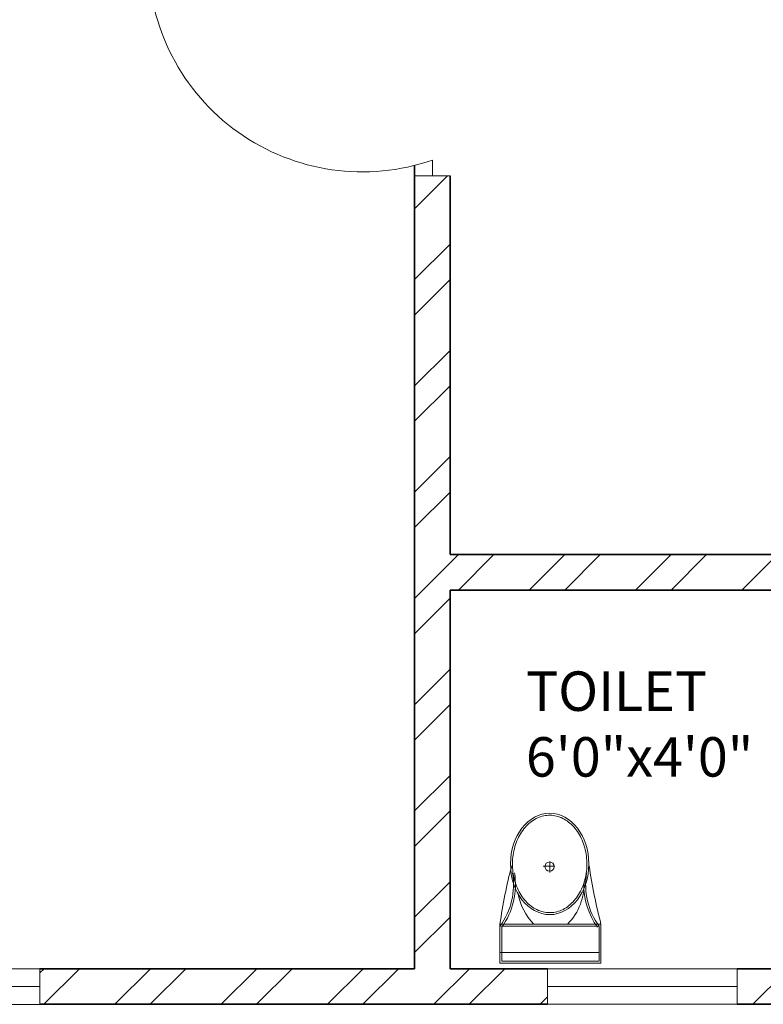
# Model space of a CAD drawing. Units: inches. Extents: x 1885 to 2748, y 783 to 2421.
# Tile 42 of 117: x 2098 to 2192, y 1558 to 1683. Entities that reach past the tile are written whole.
import ezdxf

# ---------------------------------------------------------------- set-up
doc = ezdxf.new("R2010")
doc.units = ezdxf.units.IN
for name, color, linetype, lineweight in [('A-AREA-IDEN', 7, 'Continuous', 18), ('A-DOOR', 31, 'Continuous', 18), ('A-FLOR-FIXT', 8, 'Continuous', 18), ('A-GLAZ', 181, 'Continuous', 18), ('A-WALL', 7, 'Continuous', 35)]:
    doc.layers.add(name, color=color, linetype=linetype, lineweight=lineweight)
doc.layers.add('A-WALL-PATT', color=85, linetype='Continuous', lineweight=13, true_color=0x58ba48)
doc.styles.get("Standard").update_dxf_attribs({"font": 'arial.ttf'})

# ---------------------------------------------------------------- blocks, each defined once
blk = doc.blocks.new('A$C31115884')
for p, q in [((257.5, 466.4), (257.5, 523.2)), ((283.1, 497.7), (223.4, 497.7)), ((0, 200), (0, 0)), ((520, 200), (0, 200)), ((10, 190), (10, 10)), ((510, 190), (10, 190)), ((510, 10), (510, 190)), ((520, 0), (520, 200)), ((510, 54.5), (0, 54.5)), ((10, 10), (510, 10)), ((0, 0), (520, 0))]:
    blk.add_line(p, q)
blk.add_circle((255.6, 496.4), 23.6)
for centre, radius, start, end in [((2777.7, -204.6), 2807, 165.4549, 171.7133), ((-294.5, 403.3), 364.7, 324.2091, 9.3499), ((-294.5, 403.3), 374.7, 324.2091, 9.3499), ((805.8, 403.3), 364.7, 170.6501, 215.7909), ((3237, 905), 2807, 188.2867, 194.5451), ((139.5, 406.2), 293.5, 315.8436, 2.6563), ((805.8, 403.3), 374.7, 179.2036, 215.7909), ((383.6, 406.2), 293.5, 190.2774, 224.1564)]:
    blk.add_arc(centre, radius, start, end)
blk.add_ellipse((256.2, 509.9), major_axis=(0, -260.7), ratio=0.772727)
blk.add_open_spline([(256.2, 259.2), (263.1, 259.2), (270, 259.7), (287.8, 262.3), (298.7, 265.1), (319.9, 273.1), (330.2, 278.4), (350.1, 291.1), (359.7, 298.7), (377.7, 315.9), (386.2, 325.5), (401.7, 346.6), (408.8, 358.1), (421.3, 382.5), (426.8, 395.5), (435.9, 422.4), (439.5, 436.4), (444.8, 465.1), (446.5, 479.7), (447.9, 509.2), (447.6, 524), (445, 553.3), (442.7, 567.8), (436.3, 596), (432.1, 609.7), (421.9, 636), (416, 648.6), (402.5, 672.1), (395, 683), (378.6, 703), (369.8, 712.1), (351.1, 728), (341.3, 734.8), (320.9, 746.2), (310.4, 750.7), (288.9, 757.3), (278, 759.4), (256, 761), (245, 760.6), (223.1, 757.2), (212.3, 754.3), (191.1, 746.1), (180.8, 740.7), (160.9, 727.8), (151.4, 720.1), (133.5, 702.7), (125.1, 693), (109.6, 671.7), (102.6, 660.2), (90.2, 635.7), (84.9, 622.7), (76, 595.6), (72.4, 581.6), (67.2, 552.9), (65.6, 538.2), (64.4, 508.8), (64.8, 494), (67.5, 464.7), (69.9, 450.2), (76.6, 422), (80.8, 408.3), (91.1, 382.2), (97.2, 369.7), (110.8, 346.3), (118.4, 335.4), (134.8, 315.6), (143.7, 306.7), (162.4, 290.9), (172.3, 284.2), (192.8, 273), (203.3, 268.6), (224.8, 262.2), (235.8, 260.2), (249.9, 259.3), (253, 259.2), (256.2, 259.2)], degree=3, knots=[0, 0, 0, 0, 0.110105, 0.110105, 0.285049, 0.285049, 0.459994, 0.459994, 0.634938, 0.634938, 0.809882, 0.809882, 0.984827, 0.984827, 1.159771, 1.159771, 1.334715, 1.334715, 1.50966, 1.50966, 1.684604, 1.684604, 1.859549, 1.859549, 2.034493, 2.034493, 2.209437, 2.209437, 2.384382, 2.384382, 2.559326, 2.559326, 2.73427, 2.73427, 2.909215, 2.909215, 3.084159, 3.084159, 3.259103, 3.259103, 3.434048, 3.434048, 3.608992, 3.608992, 3.783936, 3.783936, 3.958881, 3.958881, 4.133825, 4.133825, 4.30877, 4.30877, 4.483714, 4.483714, 4.658658, 4.658658, 4.833603, 4.833603, 5.008547, 5.008547, 5.183491, 5.183491, 5.358436, 5.358436, 5.53338, 5.53338, 5.708324, 5.708324, 5.883269, 5.883269, 6.058213, 6.058213, 6.233158, 6.233158, 6.283185, 6.283185, 6.283185, 6.283185])
blk = doc.blocks.new('WIN-60')
for p, q in [((0, 60), (4.5, 60)), ((0, 60), (0, 0)), ((4.5, 60), (2.25, 60)), ((2.25, 60), (2.25, 0)), ((4.5, 0), (4.5, 60)), ((2.25, 0), (0, 0)), ((0, 0), (4.5, 0))]:
    blk.add_line(p, q)
blk = doc.blocks.new('WIN-24')
for p, q in [((0, 4.5), (0, 0)), ((0, 4.5), (24, 4.5)), ((24, 2.25), (24, 4.5)), ((24, 4.5), (24, 0)), ((0, 0), (0, 2.25)), ((0, 2.25), (24, 2.25)), ((24, 0), (0, 0))]:
    blk.add_line(p, q)

msp = doc.modelspace()

# ---------------------------------------------------------------- hatches: boundary and pattern name
at = {"layer": 'A-WALL-PATT'}
h = msp.add_hatch(dxfattribs=at)
h.set_pattern_fill('ANSI32', color=256)
h.paths.add_polyline_path([(2007.77, 2318.01), (1980.77, 2318.01), (1980.77, 2281.22), (1985.27, 2281.22), (1985.27, 2313.51), (2007.77, 2313.51), (2007.77, 2315.76)])
h.paths.add_polyline_path([(2094.32, 2318.01), (2067.77, 2318.01), (2067.77, 2313.51), (2094.32, 2313.51), (2094.32, 2315.76)])
h.paths.add_polyline_path([(2131.37, 2315.76), (2131.37, 2318.01), (2131.19, 2318.01), (2112.61, 2318.01), (2112.61, 2313.51), (2117.27, 2313.51), (2117.27, 2255.2), (2121.77, 2255.2), (2121.77, 2313.51), (2131.37, 2313.51)])
h.paths.add_polyline_path([(2190.51, 2318.01), (2155.37, 2318.01), (2155.37, 2313.51), (2169.77, 2313.51), (2169.77, 2229.51), (2121.77, 2229.51), (2121.77, 2233.45), (2119.52, 2233.45), (2117.27, 2233.45), (2117.27, 2201.1), (2121.77, 2201.1), (2121.77, 2225.01), (2169.77, 2225.01), (2169.77, 2165.01), (2306.27, 2165.01), (2306.27, 2066.01), (2310.77, 2066.01), (2344.27, 2066.01), (2486.27, 2066.01), (2486.27, 1886.01), (2483.02, 1886.01), (2483.02, 1881.51), (2486.27, 1881.51), (2486.27, 1880.68), (2490.77, 1880.68), (2490.77, 2070.51), (2344.27, 2070.51), (2310.77, 2070.51), (2310.77, 2165.01), (2310.77, 2173.64), (2308.52, 2173.64), (2306.27, 2173.64), (2306.27, 2169.51), (2174.27, 2169.51), (2174.27, 2313.51), (2190.51, 2313.51), (2190.51, 2315.76)])
h.paths.add_polyline_path([(1985.27, 2221.22), (1980.77, 2221.22), (1980.77, 2165.01), (1992.77, 2165.01), (1992.77, 2141.93), (1997.27, 2141.93), (1997.27, 2165.01), (2117.27, 2165.01), (2117.27, 2163.13), (2121.77, 2163.13), (2121.77, 2172.73), (2119.52, 2172.73), (2117.27, 2172.73), (2117.27, 2169.51), (1985.27, 2169.51)])
h.paths.add_polyline_path([(1997.27, 2105.93), (1992.77, 2105.93), (1992.77, 2070.51), (2016.77, 2070.51), (2016.77, 2059.12), (2019.02, 2059.12), (2021.27, 2059.12), (2021.27, 2070.51), (2117.27, 2070.51), (2117.27, 2022.51), (2114.42, 2022.51), (2114.42, 2018.01), (2123.63, 2018.01), (2123.63, 2020.26), (2123.63, 2022.51), (2121.77, 2022.51), (2121.77, 2142.59), (2119.52, 2142.59), (2117.27, 2142.59), (2117.27, 2075.01), (1997.27, 2075.01)])
h.paths.add_polyline_path([(2092.03, 2020.26), (2092.03, 2022.51), (2021.27, 2022.51), (2021.27, 2035.12), (2016.77, 2035.12), (2016.77, 2018.01), (2016.77, 1978.78), (2021.27, 1978.78), (2021.27, 2018.01), (2092.03, 2018.01)])
h.paths.add_polyline_path([(2260.94, 2022.51), (2153.1, 2022.51), (2153.1, 2020.26), (2153.1, 2018.01), (2155.27, 2018.01), (2155.27, 1886.01), (2107.63, 1886.01), (2107.63, 1881.51), (2182.91, 1881.51), (2182.91, 1883.76), (2182.91, 1886.01), (2159.77, 1886.01), (2159.77, 2018.01), (2260.94, 2018.01), (2260.94, 2020.26)])
h.paths.add_polyline_path([(2047.63, 1883.76), (2047.63, 1886.01), (2021.27, 1886.01), (2021.27, 1918.78), (2019.02, 1918.78), (2016.77, 1918.78), (2016.77, 1881.51), (2047.63, 1881.51)])
h.paths.add_polyline_path([(2306.36, 1883.76), (2306.36, 1886.01), (2296.27, 1886.01), (2296.27, 1982.01), (2316.54, 1982.01), (2316.54, 1984.26), (2316.54, 1986.51), (2296.27, 1986.51), (2296.27, 2022.51), (2289.28, 2022.51), (2289.28, 2018.01), (2291.77, 2018.01), (2291.77, 1886.01), (2242.91, 1886.01), (2242.91, 1881.51), (2306.36, 1881.51)], flags=17)
h.paths.add_polyline_path([(1985.27, 1843.01), (2021.6, 1843.01), (2021.53, 1845.44), (2021.48, 1847.51), (1980.77, 1847.51), (1980.77, 1809.45), (1985.27, 1809.45)])
h.paths.add_polyline_path([(2131.48, 1845.26), (2131.48, 1847.51), (2081.53, 1847.51), (2081.53, 1843.01), (2117.27, 1843.01), (2117.27, 1784.15), (2119.52, 1784.15), (2121.77, 1784.15), (2121.77, 1843.01), (2131.48, 1843.01)])
h.paths.add_polyline_path([(2203.89, 1847.51), (2155.48, 1847.51), (2155.48, 1843.01), (2169.77, 1843.01), (2169.77, 1759.01), (2121.77, 1759.01), (2121.77, 1761.46), (2117.27, 1761.46), (2117.27, 1730.43), (2121.77, 1730.43), (2121.77, 1754.51), (2177.42, 1754.51), (2177.42, 1756.76), (2177.42, 1759.01), (2174.27, 1759.01), (2174.27, 1843.01), (2203.89, 1843.01)])
h.paths.add_polyline_path([(2335.55, 1845.26), (2335.55, 1847.51), (2239.89, 1847.51), (2239.89, 1843.01), (2306.27, 1843.01), (2306.27, 1759.01), (2199.49, 1759.01), (2199.49, 1754.51), (2310.77, 1754.51), (2310.77, 1843.01), (2335.55, 1843.01)])
h.paths.add_polyline_path([(2348.77, 2022.51), (2344.27, 2022.51), (2344.27, 1986.51), (2341.68, 1986.51), (2341.68, 1982.01), (2344.27, 1982.01), (2344.27, 1886.01), (2330.36, 1886.01), (2330.36, 1881.51), (2361.63, 1881.51), (2361.63, 1883.76), (2361.63, 1886.01), (2348.77, 1886.01)], flags=17)
h.paths.add_polyline_path([(2283.25, 2315.76), (2283.25, 2318.01), (2238.51, 2318.01), (2238.51, 2313.51), (2283.25, 2313.51)], flags=17)
h.paths.add_polyline_path([(2363.27, 2348.01), (2388.68, 2348.01), (2388.68, 2350.26), (2388.68, 2352.51), (2358.77, 2352.51), (2358.77, 2348.01), (2358.77, 2318.01), (2344.48, 2318.01), (2344.48, 2313.51), (2358.77, 2313.51), (2358.77, 2229.51), (2310.77, 2229.51), (2310.77, 2231.95), (2306.27, 2231.95), (2306.27, 2205.61), (2310.77, 2205.61), (2310.77, 2225.01), (2358.77, 2225.01), (2358.77, 2211.51), (2452.33, 2211.51), (2452.33, 2213.76), (2452.33, 2216.01), (2363.27, 2216.01), (2363.27, 2318.01)])
h.paths.add_polyline_path([(2310.77, 2313.51), (2320.48, 2313.51), (2320.48, 2315.76), (2320.48, 2318.01), (2302.73, 2318.01), (2302.73, 2313.51), (2306.27, 2313.51), (2306.27, 2251.08), (2310.77, 2251.08)], flags=17)
h.paths.add_polyline_path([(2490.77, 2352.51), (2486.27, 2352.51), (2448.68, 2352.51), (2448.68, 2348.01), (2486.27, 2348.01), (2486.27, 2318.01), (2486.27, 2216.01), (2481.78, 2216.01), (2481.78, 2211.51), (2486.27, 2211.51), (2486.27, 2165.01), (2493.29, 2165.01), (2493.29, 2167.26), (2493.29, 2169.51), (2490.77, 2169.51), (2490.77, 2313.51), (2494.43, 2313.51), (2494.43, 2318.01), (2490.77, 2318.01)])
h.paths.add_polyline_path([(2534.65, 2318.01), (2515.69, 2318.01), (2515.69, 2313.51), (2534.65, 2313.51), (2534.65, 2315.76)])
h.paths.add_polyline_path([(2618.27, 2318.01), (2594.65, 2318.01), (2594.65, 2313.51), (2613.77, 2313.51), (2613.77, 2281.71), (2618.27, 2281.71)])
h.paths.add_polyline_path([(2618.27, 2221.71), (2613.77, 2221.71), (2613.77, 2169.51), (2554.02, 2169.51), (2554.02, 2165.01), (2613.77, 2165.01), (2613.77, 2152.88), (2618.27, 2152.88)])
h.paths.add_polyline_path([(2618.27, 2128.88), (2616.02, 2128.88), (2613.77, 2128.88), (2613.77, 2117.01), (2529.77, 2117.01), (2529.77, 2165.01), (2532.85, 2165.01), (2532.85, 2169.51), (2522.87, 2169.51), (2522.87, 2165.01), (2525.27, 2165.01), (2525.27, 2117.01), (2525.27, 2112.51), (2525.27, 2108.58), (2529.77, 2108.58), (2529.77, 2112.51), (2613.77, 2112.51), (2613.77, 2080.19), (2618.27, 2080.19)])
h.paths.add_polyline_path([(2618.27, 2044.19), (2616.02, 2044.19), (2613.77, 2044.19), (2613.77, 2015.51), (2529.77, 2015.51), (2529.77, 2088.58), (2527.52, 2088.58), (2525.27, 2088.58), (2525.27, 2011.01), (2613.77, 2011.01), (2613.77, 1956.75), (2618.27, 1956.75)])
h.paths.add_polyline_path([(2618.27, 1881.51), (2618.27, 1896.75), (2613.77, 1896.75), (2613.77, 1881.51), (2613.77, 1847.51), (2592.71, 1847.51), (2592.71, 1843.01), (2613.77, 1843.01), (2613.77, 1765.01), (2613.77, 1760.51), (2609.62, 1760.51), (2609.62, 1756.01), (2613.77, 1756.01), (2613.77, 1660.01), (2608.54, 1660.01), (2608.54, 1655.51), (2613.77, 1655.51), (2613.77, 1508.16), (2618.27, 1508.16)])
h.paths.add_polyline_path([(2565.77, 1843.01), (2569, 1843.01), (2569, 1847.51), (2490.77, 1847.51), (2490.77, 1849.7), (2488.52, 1849.7), (2486.27, 1849.7), (2486.27, 1847.51), (2477.27, 1847.51), (2477.27, 1838.51), (2477.27, 1821.49), (2486.27, 1821.49), (2486.27, 1838.51), (2561.27, 1838.51), (2561.27, 1765.01), (2486.27, 1765.01), (2486.27, 1786.16), (2477.27, 1786.16), (2477.27, 1765.01), (2477.27, 1756.01), (2486.27, 1756.01), (2565.77, 1756.01), (2585.62, 1756.01), (2585.62, 1758.26), (2585.62, 1760.51), (2565.77, 1760.51), (2565.77, 1765.01)])
h.paths.add_polyline_path([(2486.27, 1651.01), (2561.27, 1651.01), (2561.27, 1567.01), (2486.27, 1567.01), (2486.27, 1591.32), (2477.27, 1591.32), (2477.27, 1567.01), (2477.27, 1558.01), (2477.27, 1555.44), (2481.77, 1555.44), (2481.77, 1558.01), (2568.65, 1558.01), (2568.65, 1560.26), (2568.65, 1562.51), (2565.77, 1562.51), (2565.77, 1655.51), (2584.54, 1655.51), (2584.54, 1657.76), (2584.54, 1660.01), (2565.77, 1660.01), (2486.27, 1660.01), (2477.27, 1660.01), (2477.27, 1651.01), (2477.27, 1632.99), (2486.27, 1632.99)])
h.paths.add_polyline_path([(2449.97, 1883.76), (2449.97, 1886.01), (2421.63, 1886.01), (2421.63, 1881.51), (2449.97, 1881.51)], flags=17)
h.paths.add_polyline_path([(2447.27, 1847.51), (2395.55, 1847.51), (2395.55, 1843.01), (2442.77, 1843.01), (2442.77, 1809.27), (2447.27, 1809.27)])
h.paths.add_polyline_path([(1985.27, 1749.45), (1980.77, 1749.45), (1980.77, 1694.5), (1985.27, 1694.5), (1985.27, 1694.51), (1986.9, 1694.51), (1986.9, 1697.78), (1986.9, 1699.01), (1985.27, 1699.01)])
h.paths.add_polyline_path([(2152.77, 1699.01), (2121.77, 1699.01), (2121.77, 1703.67), (2119.52, 1703.67), (2117.27, 1703.67), (2117.27, 1699.01), (2009.22, 1699.01), (2009.22, 1694.51), (2148.27, 1694.51), (2148.27, 1692.63), (2152.77, 1692.63)])
h.paths.add_polyline_path([(2016.27, 1694.51), (2011.77, 1694.51), (2011.77, 1558.01), (2040.81, 1558.01), (2040.81, 1560.26), (2040.81, 1562.51), (2016.27, 1562.51)])
h.paths.add_polyline_path([(2152.77, 1663.02), (2150.52, 1663.02), (2148.27, 1663.02), (2148.27, 1562.51), (2100.81, 1562.51), (2100.81, 1558.01), (2165.12, 1558.01), (2165.12, 1560.26), (2165.12, 1562.51), (2152.77, 1562.51), (2152.77, 1610.51), (2224.77, 1610.51), (2224.77, 1607.99), (2229.27, 1607.99), (2229.27, 1615.01), (2152.77, 1615.01)])
h.paths.add_polyline_path([(2238.61, 1560.26), (2238.61, 1562.51), (2229.27, 1562.51), (2229.27, 1588.76), (2227.02, 1588.76), (2224.77, 1588.77), (2224.77, 1562.51), (2189.12, 1562.51), (2189.12, 1558.01), (2238.61, 1558.01)])
h.paths.add_polyline_path([(2336.02, 1560.26), (2336.02, 1562.51), (2310.77, 1562.51), (2310.77, 1656.35), (2308.52, 1656.35), (2306.27, 1656.35), (2306.27, 1562.51), (2286.61, 1562.51), (2286.61, 1558.01), (2336.02, 1558.01)])
h.paths.add_polyline_path([(2447.27, 1690.97), (2445.02, 1690.97), (2442.77, 1690.97), (2442.77, 1687.01), (2306.27, 1687.01), (2306.27, 1680.75), (2310.77, 1680.75), (2310.77, 1682.51), (2442.77, 1682.51), (2442.77, 1562.51), (2396.02, 1562.51), (2396.02, 1558.01), (2447.27, 1558.01)])
h.paths.add_polyline_path([(2447.27, 1749.27), (2445.02, 1749.27), (2442.77, 1749.27), (2442.77, 1717.23), (2447.27, 1717.23)])
h.paths.add_polyline_path([(2044.67, 1521.76), (2044.67, 1524.01), (2007.27, 1524.01), (2007.27, 1503.49), (2009.52, 1503.49), (2011.77, 1503.49), (2011.77, 1519.51), (2044.67, 1519.51)])
h.paths.add_polyline_path([(2177.97, 1521.76), (2177.97, 1524.01), (2104.67, 1524.01), (2104.67, 1519.51), (2145.77, 1519.51), (2145.77, 1387.51), (2143.37, 1387.51), (2143.37, 1383.01), (2251.59, 1383.01), (2251.59, 1385.26), (2251.59, 1387.51), (2150.27, 1387.51), (2150.27, 1519.51), (2177.97, 1519.51)])
h.paths.add_polyline_path([(2298.7, 1524.01), (2237.97, 1524.01), (2237.97, 1519.51), (2282.27, 1519.51), (2282.27, 1387.51), (2279.68, 1387.51), (2279.68, 1383.01), (2286.77, 1383.01), (2286.77, 1419.01), (2312.45, 1419.01), (2312.45, 1421.26), (2312.45, 1423.51), (2286.77, 1423.51), (2286.77, 1519.51), (2298.7, 1519.51), (2298.7, 1521.72)], flags=17)
h.paths.add_polyline_path([(2361.9, 1521.76), (2361.9, 1524.01), (2322.7, 1524.01), (2322.7, 1519.51), (2334.77, 1519.51), (2334.77, 1423.51), (2331.93, 1423.51), (2331.93, 1419.01), (2334.77, 1419.01), (2334.77, 1387.51), (2334.77, 1383.23), (2339.27, 1383.23), (2339.27, 1387.51), (2339.27, 1519.51), (2361.9, 1519.51)], flags=17)
h.paths.add_polyline_path([(2447.27, 1521.76), (2447.27, 1524.01), (2421.9, 1524.01), (2421.9, 1519.51), (2447.27, 1519.51)], flags=17)
h.paths.add_polyline_path([(2481.77, 1529.6), (2479.52, 1529.6), (2477.27, 1529.6), (2477.27, 1524.01), (2474.49, 1524.01), (2474.49, 1519.51), (2477.27, 1519.51), (2477.27, 1334.51), (2296.77, 1334.51), (2296.77, 1240.51), (2160.27, 1240.51), (2160.27, 1180.51), (2112.27, 1180.51), (2112.27, 1207.69), (2110.02, 1207.69), (2107.77, 1207.69), (2107.77, 1171.61), (2112.27, 1171.61), (2112.27, 1176.01), (2160.27, 1176.01), (2160.27, 1092.01), (2144.22, 1092.01), (2144.22, 1087.51), (2189.5, 1087.51), (2189.5, 1089.76), (2189.5, 1092.01), (2164.77, 1092.01), (2164.77, 1236.01), (2296.77, 1236.01), (2296.77, 1231.91), (2301.27, 1231.91), (2301.27, 1330.01), (2481.77, 1330.01), (2481.77, 1387.51)])
h.paths.add_polyline_path([(2618.27, 1448.16), (2613.77, 1448.16), (2613.77, 1382.51), (2529.77, 1382.51), (2525.27, 1382.51), (2525.27, 1307.06), (2529.77, 1307.06), (2529.77, 1378.01), (2613.77, 1378.01), (2613.77, 1354.99), (2618.27, 1354.99)])
h.paths.add_polyline_path([(2618.27, 1318.99), (2613.77, 1318.99), (2613.77, 1281.01), (2529.77, 1281.01), (2529.77, 1283.79), (2527.52, 1283.79), (2525.27, 1283.79), (2525.27, 1228.51), (2516.79, 1228.51), (2516.79, 1224.01), (2533.48, 1224.01), (2533.48, 1226.26), (2533.48, 1228.51), (2529.77, 1228.51), (2529.77, 1276.51), (2613.77, 1276.51), (2613.77, 1266.02), (2618.27, 1266.02)])
h.paths.add_polyline_path([(2618.27, 1134.96), (2613.77, 1134.96), (2613.77, 1092.01), (2594.54, 1092.01), (2594.54, 1087.51), (2618.27, 1087.51)])
h.paths.add_polyline_path([(2534.54, 1092.01), (2509.77, 1092.01), (2509.77, 1087.51), (2534.54, 1087.51), (2534.54, 1089.76)])
h.paths.add_polyline_path([(2481.27, 1224.01), (2484.12, 1224.01), (2484.12, 1226.26), (2484.12, 1228.51), (2476.77, 1228.51), (2476.77, 1198.51), (2471.61, 1198.51), (2471.61, 1194.01), (2476.77, 1194.01), (2476.77, 1062.01), (2436.89, 1062.01), (2436.89, 1057.51), (2476.77, 1057.51), (2481.27, 1057.51), (2481.27, 1062.01), (2481.27, 1087.51), (2485.35, 1087.51), (2485.35, 1089.76), (2485.35, 1092.01), (2481.27, 1092.01), (2481.27, 1117.51)])
h.paths.add_polyline_path([(2439.9, 1198.51), (2349.27, 1198.51), (2349.27, 1194.01), (2349.27, 1180.51), (2301.27, 1180.51), (2301.27, 1201.9), (2299.02, 1201.9), (2296.77, 1201.9), (2296.77, 1172.34), (2299.02, 1172.34), (2301.27, 1172.34), (2301.27, 1176.01), (2349.27, 1176.01), (2349.27, 1092.01), (2334.45, 1092.01), (2334.45, 1087.51), (2349.27, 1087.51), (2349.27, 1057.51), (2353.77, 1057.51), (2376.89, 1057.51), (2376.89, 1059.76), (2376.89, 1062.01), (2353.77, 1062.01), (2353.77, 1087.51), (2353.77, 1180.51), (2353.77, 1194.01), (2439.9, 1194.01), (2439.9, 1196.26)])
h.paths.add_polyline_path([(2270.6, 1089.76), (2270.6, 1092.01), (2249.5, 1092.01), (2249.5, 1087.51), (2270.6, 1087.51)], flags=17)
h.paths.add_polyline_path([(2310.45, 1092.01), (2301.27, 1092.01), (2301.27, 1153.29), (2296.77, 1153.29), (2296.77, 1092.01), (2293.79, 1092.01), (2293.79, 1087.51), (2310.45, 1087.51), (2310.45, 1089.76)], flags=17)
h.paths.add_polyline_path([(2112.27, 1150.33), (2110.02, 1150.33), (2107.77, 1150.33), (2107.77, 1092.01), (2104.47, 1092.01), (2104.47, 1087.51), (2120.22, 1087.51), (2120.22, 1089.76), (2120.22, 1092.01), (2112.27, 1092.01)])
h.paths.add_polyline_path([(2082.17, 1092.01), (2058.14, 1092.01), (2058.14, 1087.51), (2082.17, 1087.51), (2082.17, 1089.76)])
h.paths.add_polyline_path([(1975.77, 1145.64), (1971.27, 1145.64), (1971.27, 1087.51), (1980.77, 1087.51), (1998.14, 1087.51), (1998.14, 1089.76), (1998.14, 1092.01), (1985.27, 1092.01), (1975.77, 1092.01)])
h.paths.add_polyline_path([(2112.27, 1244.38), (2110.02, 1244.38), (2107.77, 1244.38), (2107.77, 1240.51), (1992.27, 1240.51), (1992.27, 1271.01), (1987.77, 1271.01), (1987.77, 1240.51), (1980.77, 1240.51), (1975.77, 1240.51), (1971.27, 1240.51), (1971.27, 1205.64), (1975.77, 1205.64), (1975.77, 1236.01), (2107.77, 1236.01), (2107.77, 1233.44), (2112.27, 1233.44), (2112.27, 1236.01)])
h.paths.add_polyline_path([(2112.27, 1383.01), (2114.78, 1383.01), (2114.78, 1385.26), (2114.78, 1387.51), (2102.48, 1387.51), (2102.48, 1383.01), (2107.77, 1383.01), (2107.77, 1335.01), (2011.77, 1335.01), (2011.77, 1349.94), (2007.27, 1349.94), (2007.27, 1335.01), (1987.77, 1335.01), (1987.77, 1330.51), (1987.77, 1307.01), (1992.27, 1307.01), (1992.27, 1330.51), (2007.27, 1330.51), (2107.77, 1330.51), (2107.77, 1264.71), (2112.27, 1264.71)])
h.paths.add_polyline_path([(2077.86, 1387.51), (2011.77, 1387.51), (2011.77, 1390.04), (2009.52, 1390.04), (2007.27, 1390.04), (2007.27, 1373.94), (2011.77, 1373.94), (2011.77, 1383.01), (2077.86, 1383.01)])
h.paths.add_polyline_path([(2011.77, 1443.49), (2007.27, 1443.49), (2007.27, 1410.25), (2011.77, 1410.25)])

# ---------------------------------------------------------------- linework, layer by layer
at = {"layer": 'A-DOOR'}
for p, q in [((2150.52, 1663.02), (2150.52, 1665.02)), ((2148.27, 1663.02), (2152.77, 1663.02)), ((2152.77, 1663.02), (2150.52, 1663.02))]:
    msp.add_line(p, q, dxfattribs=at)
msp.add_arc((2141.64, 1690.63), 27.11, 180, 289.1371, dxfattribs=at)
at = {"layer": 'A-WALL'}
for p, q in [((2148.27, 1664.34), (2148.27, 1562.51)), ((2152.77, 1663.02), (2152.77, 1615.01)), ((2152.77, 1615.01), (2229.27, 1615.01)), ((2152.77, 1610.51), (2224.77, 1610.51)), ((2152.77, 1610.51), (2152.77, 1562.51)), ((2100.81, 1562.51), (2148.27, 1562.51)), ((2152.77, 1562.51), (2165.12, 1562.51)), ((2189.12, 1562.51), (2224.77, 1562.51)), ((2100.81, 1558.01), (2165.12, 1558.01)), ((2189.12, 1558.01), (2238.61, 1558.01))]:
    msp.add_line(p, q, dxfattribs=at)

# ---------------------------------------------------------------- block references
at = {"layer": 'A-FLOR-FIXT', "xscale": 0.0246256636748975, "yscale": 0.0246256636748975, "zscale": 0.0246256636748975}
msp.add_blockref('A$C31115884', (2159.07, 1563.24), dxfattribs=at)
at = {"layer": 'A-GLAZ', "extrusion": (0, 0, -1), "zscale": -1, "rotation": 90}
msp.add_blockref('WIN-60', (-2040.81, 1558), dxfattribs=at)
at = {"layer": 'A-GLAZ'}
msp.add_blockref('WIN-24', (2165.12, 1558.01), dxfattribs=at)

# ---------------------------------------------------------------- texts
at = {"layer": 'A-AREA-IDEN', "insert": (2162.37, 1600.2), "char_height": 5, "attachment_point": 1}
msp.add_mtext_dynamic_manual_height_columns('TOILET\\P6\'0"x4\'0"', width=114.2316, gutter_width=12.5, heights=[0], dxfattribs=at)

doc.saveas('drawing.dxf')
